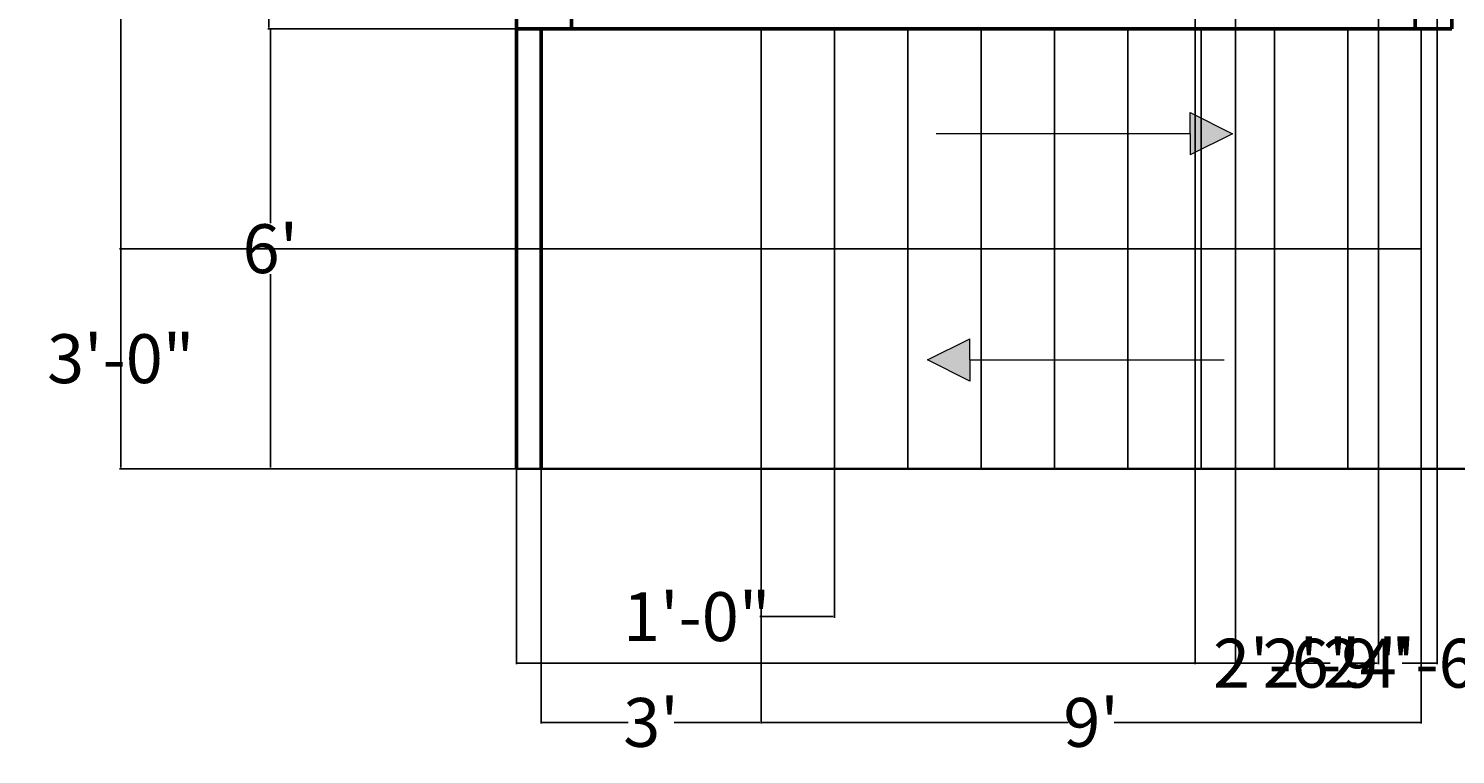
# Model space of a CAD drawing. Units: inches. Extents: x 1305 to 1889, y -508 to -5.
# Tile 1 of 8: x 1314 to 1548, y -508 to -389. Entities that reach past the tile are written whole.
import ezdxf

# ---------------------------------------------------------------- set-up
doc = ezdxf.new("R2010")
doc.units = ezdxf.units.IN
doc.header["$MEASUREMENT"] = 0
for name, color, linetype, lineweight in [('A-ANNO-DIMS', 2, 'Continuous', 18), ('A-ANNO-SYMB', 7, 'Continuous', 18), ('A-FLOR', 7, 'Continuous', 35), ('A-FLOR-STRS', 7, 'Continuous', 25), ('A-WALL', 7, 'Continuous', 50)]:
    doc.layers.add(name, color=color, linetype=linetype, lineweight=lineweight)
doc.styles.get("Standard").update_dxf_attribs({"font": 'arial.ttf', "height": 8})
doc.dimstyles.get("Standard").update_dxf_attribs({"dimtxt": 0.18, "dimasz": 0.18, "dimexe": 0.18, "dimexo": 0.0625, "dimgap": 0.09, "dimtad": 0, "dimtih": 1, "dimtoh": 1, "dimzin": 0, "dimdsep": 46, "dimlunit": 4, "dimtxsty": 'Standard', "dimcen": 0.09, "dimadec": 0, "dimazin": 0, "dimtfac": 1, "dimtofl": 0, "dimtmove": 0, "dimatfit": 3, "dimfxl": 1, "dimtolj": 1, "dimtzin": 0, "dimarcsym": 0})

# ---------------------------------------------------------------- blocks, each defined once
blk = doc.blocks.new('*D21')
at = {"layer": 'A-ANNO-DIMS', "color": 0, "lineweight": -2, "transparency": 16777216}
for p, q in [((1394.01, -244.98), (1353.36, -244.98)), ((1353.54, -245.16), (1353.54, -307.6)), ((1353.54, -389.06), (1353.54, -326.62)), ((1394.01, -389.24), (1353.36, -389.24))]:
    blk.add_line(p, q, dxfattribs=at)
at = {"layer": 'A-ANNO-DIMS', "color": 0, "transparency": 16777216}
for points in [[(1353.51, -245.16), (1353.57, -245.16), (1353.54, -244.98)], [(1353.51, -389.06), (1353.57, -389.06), (1353.54, -389.24)]]:
    blk.add_solid(points, dxfattribs=at)
at = {"layer": 'Defpoints', "color": 0, "transparency": 16777216}
for p in [(1394.07, -244.98), (1353.54, -389.24), (1394.07, -389.24)]:
    blk.add_point(p, dxfattribs=at)
at = {"layer": 'A-ANNO-DIMS', "color": 0, "transparency": 16777216, "insert": (1353.54, -317.11), "char_height": 8, "attachment_point": 5}
blk.add_mtext('\\A1;12\'-0{\\H1x;\\S1/4;}"', dxfattribs=at)
blk = doc.blocks.new('*D22')
at = {"layer": 'A-ANNO-DIMS', "color": 0, "lineweight": -2, "transparency": 16777216}
for p, q in [((1394.01, -389.24), (1353.61, -389.24)), ((1353.79, -389.42), (1353.79, -421.06)), ((1353.79, -461.06), (1353.79, -429.41)), ((1394.01, -461.24), (1353.61, -461.24))]:
    blk.add_line(p, q, dxfattribs=at)
at = {"layer": 'A-ANNO-DIMS', "color": 0, "transparency": 16777216}
for points in [[(1353.76, -389.42), (1353.82, -389.42), (1353.79, -389.24)], [(1353.76, -461.06), (1353.82, -461.06), (1353.79, -461.24)]]:
    blk.add_solid(points, dxfattribs=at)
at = {"layer": 'Defpoints', "color": 0, "transparency": 16777216}
for p in [(1394.07, -389.24), (1353.79, -461.24), (1394.07, -461.24)]:
    blk.add_point(p, dxfattribs=at)
at = {"layer": 'A-ANNO-DIMS', "color": 0, "transparency": 16777216, "insert": (1353.79, -425.24), "char_height": 8, "attachment_point": 5}
blk.add_mtext("\\A1;6'", dxfattribs=at)
blk = doc.blocks.new('*D23')
at = {"layer": 'A-ANNO-DIMS', "color": 0, "lineweight": -2, "transparency": 16777216}
for p, q in [((1398.07, -461.3), (1398.07, -502.95)), ((1434.07, -461.3), (1434.07, -502.95)), ((1398.25, -502.77), (1412.31, -502.77)), ((1433.89, -502.77), (1419.84, -502.77))]:
    blk.add_line(p, q, dxfattribs=at)
at = {"layer": 'A-ANNO-DIMS', "color": 0, "transparency": 16777216}
for points in [[(1398.25, -502.74), (1398.25, -502.8), (1398.07, -502.77)], [(1433.89, -502.74), (1433.89, -502.8), (1434.07, -502.77)]]:
    blk.add_solid(points, dxfattribs=at)
at = {"layer": 'Defpoints', "color": 0, "transparency": 16777216}
for p in [(1398.07, -461.24), (1434.07, -461.24), (1434.07, -502.77)]:
    blk.add_point(p, dxfattribs=at)
at = {"layer": 'A-ANNO-DIMS', "color": 0, "transparency": 16777216, "insert": (1416.07, -502.77), "char_height": 8, "attachment_point": 5}
blk.add_mtext("\\A1;3'", dxfattribs=at)
blk = doc.blocks.new('*D24')
at = {"layer": 'A-ANNO-DIMS', "color": 0, "lineweight": -2, "transparency": 16777216}
for p, q in [((1434.07, -461.3), (1434.07, -502.95)), ((1542.07, -461.3), (1542.07, -502.95)), ((1434.25, -502.77), (1484.3, -502.77)), ((1541.89, -502.77), (1491.85, -502.77))]:
    blk.add_line(p, q, dxfattribs=at)
at = {"layer": 'A-ANNO-DIMS', "color": 0, "transparency": 16777216}
for points in [[(1434.25, -502.74), (1434.25, -502.8), (1434.07, -502.77)], [(1541.89, -502.74), (1541.89, -502.8), (1542.07, -502.77)]]:
    blk.add_solid(points, dxfattribs=at)
at = {"layer": 'Defpoints', "color": 0, "transparency": 16777216}
for p in [(1434.07, -461.24), (1542.07, -461.24), (1542.07, -502.77)]:
    blk.add_point(p, dxfattribs=at)
at = {"layer": 'A-ANNO-DIMS', "color": 0, "transparency": 16777216, "insert": (1488.07, -502.77), "char_height": 8, "attachment_point": 5}
blk.add_mtext("\\A1;9'", dxfattribs=at)
blk = doc.blocks.new('STAIR-DIRECTION-ARROW')
h = blk.add_hatch(color=256)
h.dxf.hatch_style = 1
h.paths.add_polyline_path([(6.93, 6.93), (0, 3.46), (6.93, 0), (6.93, 3.46)])
for p, q in [((0, 3.46), (6.93, 6.93)), ((6.93, 3.46), (6.93, 6.93)), ((6.93, 0), (0, 3.46)), ((6.93, 3.46), (6.93, 0)), ((6.93, 3.46), (48.49, 3.46))]:
    blk.add_line(p, q)
blk = doc.blocks.new('*D50')
at = {"layer": 'A-ANNO-DIMS', "color": 0, "lineweight": -2, "transparency": 16777216}
for p, q in [((1394.07, -461.3), (1394.07, -493.26)), ((1688.05, -461.36), (1688.05, -493.26)), ((1394.25, -493.08), (1527.16, -493.08)), ((1687.87, -493.08), (1554.96, -493.08))]:
    blk.add_line(p, q, dxfattribs=at)
at = {"layer": 'A-ANNO-DIMS', "color": 0, "transparency": 16777216}
for points in [[(1394.25, -493.05), (1394.25, -493.11), (1394.07, -493.08)], [(1687.87, -493.05), (1687.87, -493.11), (1688.05, -493.08)]]:
    blk.add_solid(points, dxfattribs=at)
at = {"layer": 'Defpoints', "color": 0, "transparency": 16777216}
for p in [(1394.07, -461.24), (1688.05, -461.3), (1688.05, -493.08)]:
    blk.add_point(p, dxfattribs=at)
at = {"layer": 'A-ANNO-DIMS', "color": 0, "transparency": 16777216, "insert": (1541.06, -493.08), "char_height": 8, "attachment_point": 5}
blk.add_mtext('\\A1;24\'-6"', dxfattribs=at)
blk = doc.blocks.new('*D51')
at = {"layer": 'A-ANNO-DIMS', "color": 0, "lineweight": -2, "transparency": 16777216}
for p, q in [((1394.01, -110.24), (1329.13, -110.24)), ((1329.31, -110.42), (1329.31, -281.56)), ((1329.31, -461.06), (1329.31, -289.92)), ((1394.01, -461.24), (1329.13, -461.24))]:
    blk.add_line(p, q, dxfattribs=at)
at = {"layer": 'A-ANNO-DIMS', "color": 0, "transparency": 16777216}
for points in [[(1329.28, -110.42), (1329.34, -110.42), (1329.31, -110.24)], [(1329.28, -461.06), (1329.34, -461.06), (1329.31, -461.24)]]:
    blk.add_solid(points, dxfattribs=at)
at = {"layer": 'Defpoints', "color": 0, "transparency": 16777216}
for p in [(1394.07, -110.24), (1329.31, -461.24), (1394.07, -461.24)]:
    blk.add_point(p, dxfattribs=at)
at = {"layer": 'A-ANNO-DIMS', "color": 0, "transparency": 16777216, "insert": (1329.31, -285.74), "char_height": 8, "attachment_point": 5}
blk.add_mtext('\\A1;29\'-3"', dxfattribs=at)
blk = doc.blocks.new('*D55')
at = {"layer": 'A-ANNO-DIMS', "color": 0, "lineweight": -2, "transparency": 16777216}
for p, q in [((1511.68, -135.63), (1511.68, -493.26)), ((1544.68, -146.13), (1544.68, -493.26)), ((1511.86, -493.08), (1517.39, -493.08)), ((1544.5, -493.08), (1538.97, -493.08))]:
    blk.add_line(p, q, dxfattribs=at)
at = {"layer": 'A-ANNO-DIMS', "color": 0, "transparency": 16777216}
for points in [[(1511.86, -493.05), (1511.86, -493.11), (1511.68, -493.08)], [(1544.5, -493.05), (1544.5, -493.11), (1544.68, -493.08)]]:
    blk.add_solid(points, dxfattribs=at)
at = {"layer": 'Defpoints', "color": 0, "transparency": 16777216}
for p in [(1511.68, -135.57), (1544.68, -146.07), (1544.68, -493.08)]:
    blk.add_point(p, dxfattribs=at)
at = {"layer": 'A-ANNO-DIMS', "color": 0, "transparency": 16777216, "insert": (1528.18, -493.08), "char_height": 8, "attachment_point": 5}
blk.add_mtext('\\A1;2\'-9"', dxfattribs=at)
blk = doc.blocks.new('*D61')
at = {"layer": 'A-ANNO-DIMS', "color": 0, "lineweight": -2, "transparency": 16777216}
for p, q in [((1505.07, -290.3), (1505.07, -493.26)), ((1535.07, -290.3), (1535.07, -493.26)), ((1505.25, -493.08), (1509.28, -493.08)), ((1534.89, -493.08), (1530.87, -493.08))]:
    blk.add_line(p, q, dxfattribs=at)
at = {"layer": 'A-ANNO-DIMS', "color": 0, "transparency": 16777216}
for points in [[(1505.25, -493.05), (1505.25, -493.11), (1505.07, -493.08)], [(1534.89, -493.05), (1534.89, -493.11), (1535.07, -493.08)]]:
    blk.add_solid(points, dxfattribs=at)
at = {"layer": 'Defpoints', "color": 0, "transparency": 16777216}
for p in [(1505.07, -290.24), (1535.07, -290.24), (1535.07, -493.08)]:
    blk.add_point(p, dxfattribs=at)
at = {"layer": 'A-ANNO-DIMS', "color": 0, "transparency": 16777216, "insert": (1520.07, -493.08), "char_height": 8, "attachment_point": 5}
blk.add_mtext('\\A1;2\'-6"', dxfattribs=at)
blk = doc.blocks.new('*D71')
at = {"layer": 'A-ANNO-DIMS', "color": 0, "lineweight": -2, "transparency": 16777216}
for p, q in [((1434.07, -461.3), (1434.07, -485.64)), ((1446.07, -461.3), (1446.07, -485.64)), ((1434.07, -485.46), (1433.89, -485.46)), ((1445.89, -485.46), (1434.25, -485.46))]:
    blk.add_line(p, q, dxfattribs=at)
at = {"layer": 'A-ANNO-DIMS', "color": 0, "transparency": 16777216}
for points in [[(1434.25, -485.43), (1434.25, -485.49), (1434.07, -485.46)], [(1445.89, -485.43), (1445.89, -485.49), (1446.07, -485.46)]]:
    blk.add_solid(points, dxfattribs=at)
at = {"layer": 'Defpoints', "color": 0, "transparency": 16777216}
for p in [(1434.07, -461.24), (1446.07, -461.24), (1434.07, -485.46)]:
    blk.add_point(p, dxfattribs=at)
at = {"layer": 'A-ANNO-DIMS', "color": 0, "transparency": 16777216, "insert": (1423.55, -485.46), "char_height": 8, "attachment_point": 5}
blk.add_mtext('\\A1;1\'-0"', dxfattribs=at)
blk = doc.blocks.new('*D72')
at = {"layer": 'A-ANNO-DIMS', "color": 0, "lineweight": -2, "transparency": 16777216}
for p, q in [((1434.01, -425.24), (1329.13, -425.24)), ((1329.31, -425.42), (1329.31, -439.06)), ((1329.31, -461.06), (1329.31, -447.42)), ((1434.01, -461.24), (1329.13, -461.24))]:
    blk.add_line(p, q, dxfattribs=at)
at = {"layer": 'A-ANNO-DIMS', "color": 0, "transparency": 16777216}
for points in [[(1329.28, -425.42), (1329.34, -425.42), (1329.31, -425.24)], [(1329.28, -461.06), (1329.34, -461.06), (1329.31, -461.24)]]:
    blk.add_solid(points, dxfattribs=at)
at = {"layer": 'Defpoints', "color": 0, "transparency": 16777216}
for p in [(1329.31, -425.24), (1434.07, -425.24), (1434.07, -461.24)]:
    blk.add_point(p, dxfattribs=at)
at = {"layer": 'A-ANNO-DIMS', "color": 0, "transparency": 16777216, "insert": (1329.31, -443.24), "char_height": 8, "attachment_point": 5}
blk.add_mtext('\\A1;3\'-0"', dxfattribs=at)

msp = doc.modelspace()

# ---------------------------------------------------------------- linework, layer by layer
at = {"layer": 'A-ANNO-DIMS'}
msp.add_line((1394.074, -389.239), (1353.535, -389.239), dxfattribs=at)
at = {"layer": 'A-FLOR'}
msp.add_line((1394.074, -461.239), (1637.526, -461.239), dxfattribs=at)
at = {"layer": 'A-FLOR-STRS'}
for p, q in [((1434.074, -389.239), (1434.074, -461.239)), ((1446.074, -389.239), (1446.074, -461.239)), ((1458.074, -389.239), (1458.074, -461.239)), ((1470.074, -389.239), (1470.074, -461.239)), ((1482.074, -389.239), (1482.074, -461.239)), ((1494.074, -389.239), (1494.074, -461.239)), ((1506.074, -389.239), (1506.074, -461.239)), ((1518.074, -389.239), (1518.074, -461.239)), ((1530.074, -389.239), (1530.074, -461.239)), ((1542.074, -389.239), (1542.074, -461.239)), ((1434.074, -425.239), (1542.074, -425.239))]:
    msp.add_line(p, q, dxfattribs=at)
at = {"layer": 'A-WALL'}
for p, q in [((1394.074, -110.239), (1394.074, -461.239)), ((1403.074, -110.239), (1403.074, -389.239)), ((1541.074, -248.321), (1541.074, -389.239)), ((1547.074, -248.321), (1547.074, -389.239)), ((1394.074, -389.239), (1547.074, -389.239)), ((1398.074, -389.239), (1398.074, -461.239))]:
    msp.add_line(p, q, dxfattribs=at)

# ---------------------------------------------------------------- block references
at = {"layer": 'A-ANNO-SYMB', "rotation": 180}
msp.add_blockref('STAIR-DIRECTION-ARROW', (1511.211, -402.967), dxfattribs=at)
at = {"layer": 'A-ANNO-SYMB'}
msp.add_blockref('STAIR-DIRECTION-ARROW', (1461.322, -446.91), dxfattribs=at)

# ---------------------------------------------------------------- dimensions: what is measured, and where the dimension line sits
at = {"layer": 'A-ANNO-DIMS'}
for base, p1, p2, angle, override, picture, middle in [((1329.31, -461.239), (1394.074, -110.239), (1394.074, -461.239), 90, {"dimdec": 1, "dimlfac": 1, "dimrnd": 0, "dimzin": 1, "dimdsep": 46, "dimlunit": 4, "dimfrac": 2}, '*D51', (1329.31, -285.739)), ((1353.535, -389.239), (1394.074, -244.978), (1394.074, -389.239), 90, {"dimclrd": 0, "dimclre": 0, "dimclrt": 0}, '*D21', (1353.535, -317.108)), ((1353.792, -461.239), (1394.074, -389.239), (1394.074, -461.239), 90, {"dimclrd": 0, "dimclre": 0, "dimclrt": 0}, '*D22', (1353.792, -425.239)), ((1329.31, -425.239), (1434.074, -461.239), (1434.074, -425.239), 90, {"dimdec": 1, "dimlfac": 1, "dimrnd": 0, "dimzin": 1, "dimdsep": 46, "dimlunit": 4, "dimfrac": 2}, '*D72', (1329.31, -443.239)), ((1434.074, -485.464), (1446.074, -461.239), (1434.074, -461.239), 180, {"dimdec": 1, "dimlfac": 1, "dimrnd": 0, "dimzin": 1, "dimdsep": 46, "dimlunit": 4, "dimfrac": 2}, '*D71', (1423.548, -485.464))]:
    dim = msp.add_linear_dim(base=base, p1=p1, p2=p2, angle=angle, dimstyle='Standard', override=override, dxfattribs=at)
    dim.commit()
    dim.dimension.update_dxf_attribs({"geometry": picture, "text_midpoint": middle})
for base, p1, p2, override, picture, middle in [((1544.679, -493.076), (1511.679, -135.569), (1544.679, -146.069), {"dimdec": 1, "dimlfac": 1, "dimrnd": 0, "dimzin": 1, "dimdsep": 46, "dimlunit": 4, "dimfrac": 2}, '*D55', (1528.179, -493.076)), ((1535.074, -493.076), (1505.074, -290.239), (1535.074, -290.239), {"dimdec": 1, "dimlfac": 1, "dimrnd": 0, "dimzin": 1, "dimdsep": 46, "dimlunit": 4, "dimfrac": 2}, '*D61', (1520.074, -493.076)), ((1688.053, -493.076), (1394.074, -461.239), (1688.053, -461.295), {"dimdec": 1, "dimlfac": 1, "dimrnd": 0, "dimzin": 1, "dimdsep": 46, "dimlunit": 4, "dimfrac": 2}, '*D50', (1541.064, -493.076)), ((1434.074, -502.767), (1398.074, -461.239), (1434.074, -461.239), {"dimclrd": 0, "dimclre": 0, "dimclrt": 0}, '*D23', (1416.074, -502.767)), ((1542.074, -502.767), (1434.074, -461.239), (1542.074, -461.239), {"dimclrd": 0, "dimclre": 0, "dimclrt": 0}, '*D24', (1488.074, -502.767))]:
    dim = msp.add_linear_dim(base=base, p1=p1, p2=p2, dimstyle='Standard', override=override, dxfattribs=at)
    dim.commit()
    dim.dimension.update_dxf_attribs({"geometry": picture, "text_midpoint": middle})

doc.saveas('drawing.dxf')
